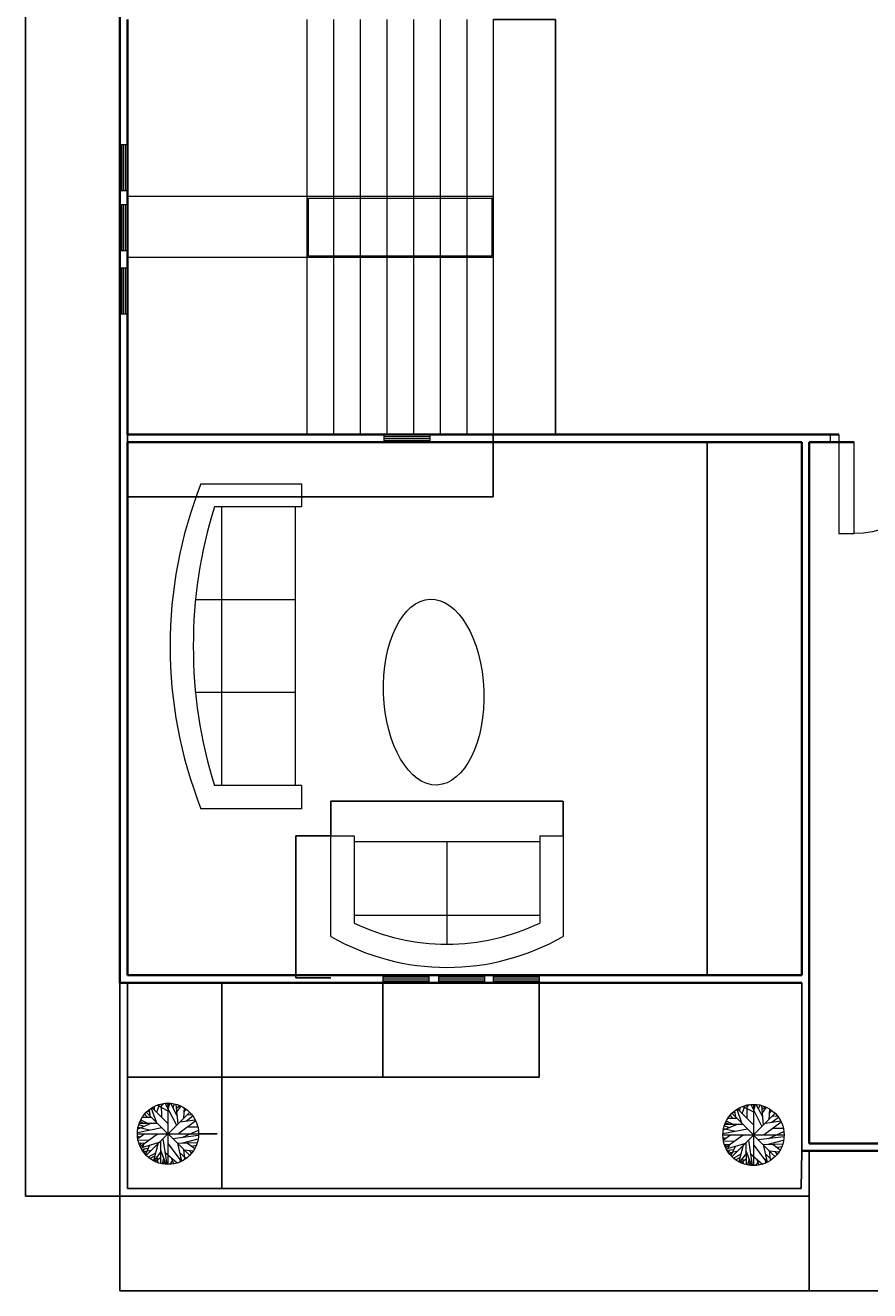
# Model space of a CAD drawing. Units: millimetres. Extents: x 1194 to 22780, y 83 to 13378.
# Tile 4 of 6: x 12489 to 18030, y 136 to 8443. Entities that reach past the tile are written whole.
import ezdxf

# ---------------------------------------------------------------- set-up
doc = ezdxf.new("R2010")
doc.units = ezdxf.units.MM
for name, color, linetype, lineweight in [('A-ANNO-DIMS', 2, 'Continuous', 18), ('A-DOOR', 3, 'Continuous', 18), ('A-FLOR-STRS', 7, 'Continuous', 18), ('A-FURN', 8, 'Continuous', 18), ('A-GLAZ', 4, 'Continuous', 18), ('A-WALL', 7, 'Continuous', 35), ('A-WALL-PRPT', 7, 'Continuous', 25), ('L-PLNT', 3, 'Continuous', 13)]:
    doc.layers.add(name, color=color, linetype=linetype, lineweight=lineweight)
doc.styles.get("Standard").update_dxf_attribs({"font": 'arial.ttf'})
doc.dimstyles.get("Standard").update_dxf_attribs({"dimtxt": 0.18, "dimasz": 0.18, "dimexe": 0.18, "dimexo": 0.0625, "dimgap": 0.09, "dimtad": 0, "dimtih": 1, "dimtoh": 1, "dimdec": 4, "dimzin": 0, "dimdsep": 46, "dimtxsty": 'Standard', "dimcen": 0.09, "dimadec": 0, "dimazin": 0, "dimtfac": 1, "dimtdec": 4, "dimtofl": 0, "dimtmove": 0, "dimatfit": 3, "dimfxl": 1, "dimtolj": 1, "dimtzin": 0, "dimarcsym": 0})

# ---------------------------------------------------------------- blocks, each defined once
blk = doc.blocks.new('Window - Wood Frame 36 in. Wide plan')
for p, q in [((0, 6), (0, 0)), ((0, 4.5), (36, 4.5)), ((0, 3), (36, 3)), ((0, 1.5), (36, 1.5)), ((36, 6), (36, 0))]:
    blk.add_line(p, q)
blk = doc.blocks.new('Sofa - Roundback 7 ft.')
for p, q in [((-12.00002, -32.4421), (-12.00003, -6.5971)), ((11.99997, -32.4421), (11.99998, -6.5971)), ((-36.000027, -34), (-36.000027, -11.4696)), ((35.99998, -34), (35.99998, -11.4696)), ((-35.999844, -13.3819), (35.9998, -13.3819)), ((-36.000027, -32.4421), (35.99998, -32.4421))]:
    blk.add_line(p, q)
for points in [[(-36.000027, -34), (-42.000027, -34), (-42.000027, -8)], [(41.99998, -8), (41.99998, -34), (35.99998, -34)]]:
    blk.add_lwpolyline(points)
for centre, radius, start, end in [((0, -114.25), 114.25, 68.43141, 111.5686), ((-0.00001, -127.1968), 121.1968, 72.72033, 107.2797)]:
    blk.add_arc(centre, radius, start, end)
blk = doc.blocks.new('Sofa - Roundback Loveseat 5 ft.')
for p, q in [((0, -32.44198), (0, -5.99998)), ((-24, -33.99998), (-24, -11.46958)), ((24.00004, -33.99998), (24.00004, -11.46958)), ((-23.9998, -13.38178), (23.99986, -13.38178)), ((-24, -32.44198), (24.00004, -32.44198))]:
    blk.add_line(p, q)
for points in [[(-24, -33.99998), (-30, -33.99998), (-30, -7.99998)], [(30.00004, -7.99998), (30.00004, -33.99998), (24.00004, -33.99998)]]:
    blk.add_lwpolyline(points)
for centre, radius, start, end in [((0, -60.24998), 60.24998, 60.13715, 119.8628), ((0, -61.38438), 55.38444, 64.32083, 115.6792)]:
    blk.add_arc(centre, radius, start, end)
blk = doc.blocks.new('Tree - deciduous plan')
for p, q in [((-32.6092, 50.4264), (-23.2782, 23.5674)), ((-31.2008, 51.1035), (-0.2149, 20.1818)), ((-26.4472, 46.5894), (-26.2712, 53.8116)), ((-22.0458, 42.0753), (-16.5881, 57.6486)), ((-21.1656, 55.8436), (-0.0388, 45.0094)), ((-12.5388, 54.9406), (-7.9613, 59.4546)), ((-12.3627, 32.1443), (-12.5388, 58.7776)), ((-5.3205, 59.6806), (16.5105, 16.7963)), ((2.426, 54.9406), (-1.4472, 59.9056)), ((0, 59.9996), (0, -60)), ((0.4894, 48.6208), (3.6584, 59.6806)), ((18.2711, 35.5298), (5.419, 59.6806)), ((9.8203, 51.5549), (12.8133, 58.5516)), ((19.6795, 19.5047), (16.3344, 57.6486)), ((17.0387, 51.1035), (23.2006, 55.1666)), ((17.7429, 43.6552), (25.4894, 54.2636)), ((31.6513, 50.8778), (30.2429, 30.5643)), ((-53.2078, 27.4044), (-40.1797, 20.859)), ((-49.8627, 32.8214), (-32.7853, 32.8214)), ((-45.8134, 38.2383), (-40.5318, 33.0471)), ((-43.8768, 36.4326), (-44.405, 40.2696)), ((42, 42), (-42, -42)), ((42, -42), (-42, 42)), ((-40.1797, 44.558), (-36.4825, 43.2038)), ((-37.0107, 47.0408), (-35.25, 35.5298)), ((54.3626, 25.3731), (20.9119, 0.3198)), ((23.3767, 23.3417), (53.3063, 27.4044)), ((31.1232, 42.5267), (35.8767, 48.1693)), ((36.2288, 25.1474), (48.9049, 35.0784)), ((37.1091, 37.1098), (46.6161, 37.5612)), ((-59.7219, 2.8025), (-12.0106, 12.0565)), ((-32.2571, 20.6333), (-59.1937, 9.348)), ((-58.6656, 12.7336), (-35.9543, 7.5424)), ((-57.081, 17.9248), (-47.0458, 14.7649)), ((-56.0247, 20.859), (-20.8134, 20.859)), ((-54.7923, 24.4702), (-47.75, 21.0847)), ((-54.6162, -24.7335), (-20.2853, 0.0941)), ((29.3626, -6.6771), (59.4682, 7.091)), ((38.5175, 13.4107), (58.2359, 13.6364)), ((-60, 0), (60, 0)), ((-59.7219, -4.8714), (-54.2641, -6.6771)), ((-45.2853, -0.1316), (-59.0177, -10.0627)), ((-58.4895, -12.3197), (-36.4825, -11.6426)), ((-57.081, -18.4138), (-45.2853, -17.9624)), ((-52.6797, -18.188), (-55.4966, -22.0251)), ((-53.2078, -27.442), (-16.7641, -16.6081)), ((-47.2219, -19.3166), (-50.2148, -26.3135)), ((-35.9543, -22.4765), (-44.0529, -40.5329)), ((-19.9331, -20.2194), (-28.5599, -52.721)), ((-14.8275, -15.0282), (-14.6515, -57.6865)), ((-10.074, -10.0627), (-2.5036, -59.7178)), ((-0.0388, -19.0909), (25.8415, -53.8495)), ((9.2922, -9.1598), (59.6443, -2.8401)), ((18.6232, -18.6394), (26.7218, -53.3981)), ((18.7992, -18.6394), (57.3556, -17.2853)), ((26.3697, -18.4138), (58.9401, -9.8369)), ((38.1654, -18.188), (52.426, -29.0219)), ((45.9119, -24.0564), (55.595, -22.2508)), ((-38.9472, -29.0219), (-51.4472, -30.6018)), ((-46.5177, -30.1504), (-49.5106, -33.536)), ((-32.4331, -32.4075), (-48.1021, -35.5674)), ((-43.7008, -34.6645), (-46.6937, -37.373)), ((-24.6867, -37.8244), (-38.7712, -45.7241)), ((-26.2712, -43.9185), (-34.7219, -48.6583)), ((-14.6515, -36.2445), (-27.6797, -52.9467)), ((-14.6515, -47.3041), (-25.0388, -54.3009)), ((-21.5177, -45.4984), (-19.9331, -56.1065)), ((-14.6515, -32.1818), (-3.912, -59.4922)), ((-8.4895, -47.5298), (-11.4825, -58.5893)), ((-6.2008, -36.2445), (17.919, -57.0094)), ((5.9471, -46.6269), (10.5246, -58.5893)), ((22.8485, -36.4702), (35.3485, -48.4326)), ((24.7852, -44.8213), (23.0246, -54.978)), ((30.419, -30.1504), (32.3556, -50.0125)), ((31.4753, -31.279), (49.6091, -33.3103)), ((41.5105, -32.6332), (46.088, -38.0501)), ((-6.3768, -52.721), (-9.3698, -58.815)), ((8.4119, -53.1724), (3.8344, -59.4922))]:
    blk.add_line(p, q)
blk.add_circle((0, 0), 60)
blk = doc.blocks.new('DOOR-SWING-600')
for p, q in [((0, 0), (0, 600)), ((0, 600), (100, 600)), ((100, 600), (100, 0))]:
    blk.add_line(p, q)
blk.add_arc((100, 0), 600, 0, 90)
blk = doc.blocks.new('STAIR-DUPLEX-FLIGHT')
for p, q in [((1177, 2725.9), (1177, 0)), ((1351.8, 2725.9), (1351.8, 0)), ((1526.7, 2725.9), (1526.7, 0)), ((1701.5, 2725.9), (1701.5, 0)), ((1876.4, 2725.9), (1876.4, 0)), ((2051.2, 2725.9), (2051.2, 0)), ((2226.1, 2725.9), (2226.1, 0)), ((2400.9, 2725.9), (2400.9, 0)), ((1177, 1562.9), (0, 1562.9)), ((2400.9, 1562.9), (1177, 1562.9)), ((1187, 1552.9), (2390.9, 1552.9)), ((1187, 1172.9), (1187, 1552.9)), ((2390.9, 1552.9), (2390.9, 1172.9)), ((2400.9, 1362.9), (2400.9, 1562.9)), ((2390.9, 1172.9), (1187, 1172.9)), ((2400.9, 1162.9), (0, 1162.9))]:
    blk.add_line(p, q)
blk = doc.blocks.new('*D33')
at = {"layer": 'A-ANNO-DIMS', "color": 0, "lineweight": -2, "transparency": 16777216}
for p, q in [((14493.6, 3121.8), (14493.6, 3350.5)), ((14493.8, 3350.4), (15254.3, 3350.4)), ((16017.4, 3350.4), (15257, 3350.4)), ((16017.6, 3121.8), (16017.6, 3350.5))]:
    blk.add_line(p, q, dxfattribs=at)
at = {"layer": 'A-ANNO-DIMS', "color": 0, "transparency": 16777216}
for points in [[(14493.8, 3350.4), (14493.8, 3350.3), (14493.6, 3350.4)], [(16017.4, 3350.4), (16017.4, 3350.3), (16017.6, 3350.4)]]:
    blk.add_solid(points, dxfattribs=at)
at = {"layer": 'Defpoints', "color": 0, "transparency": 16777216}
for p in [(14493.6, 3350.4), (14493.6, 3121.8), (16017.6, 3121.8)]:
    blk.add_point(p, dxfattribs=at)
at = {"layer": 'A-ANNO-DIMS', "color": 0, "transparency": 16777216, "insert": (15255.6, 3350.4), "char_height": 0.18, "attachment_point": 5}
blk.add_mtext('\\A1;LOVESEAT 1524 TYP.', dxfattribs=at)
blk = doc.blocks.new('*D34')
at = {"layer": 'A-ANNO-DIMS', "color": 0, "lineweight": -2, "transparency": 16777216}
for p, q in [((14493.6, 3121.8), (14264.8, 3121.8)), ((14265, 3121.6), (14265, 2656.3)), ((14265, 2190.6), (14265, 2655.9)), ((14493.6, 2190.4), (14264.8, 2190.4))]:
    blk.add_line(p, q, dxfattribs=at)
at = {"layer": 'A-ANNO-DIMS', "color": 0, "transparency": 16777216}
for points in [[(14265, 3121.6), (14265, 3121.6), (14265, 3121.8)], [(14265, 2190.6), (14265, 2190.6), (14265, 2190.4)]]:
    blk.add_solid(points, dxfattribs=at)
at = {"layer": 'Defpoints', "color": 0, "transparency": 16777216}
for p in [(14493.6, 3121.8), (14265, 2190.4), (14493.6, 2190.4)]:
    blk.add_point(p, dxfattribs=at)
at = {"layer": 'A-ANNO-DIMS', "color": 0, "transparency": 16777216, "insert": (14265, 2656.1), "char_height": 0.18, "attachment_point": 5}
blk.add_mtext('\\A1;931 TYP.', dxfattribs=at)
blk = doc.blocks.new('*D39')
at = {"layer": 'A-ANNO-DIMS', "color": 0, "lineweight": -2, "transparency": 16777216}
for p, q in [((15560.2, 8481.6), (15969.2, 8481.6)), ((15969, 8481.5), (15969, 7118.9)), ((15969, 5756), (15969, 7118.5)), ((15560.2, 5755.8), (15969.2, 5755.8))]:
    blk.add_line(p, q, dxfattribs=at)
at = {"layer": 'A-ANNO-DIMS', "color": 0, "transparency": 16777216}
for points in [[(15969, 8481.5), (15969, 8481.5), (15969, 8481.6)], [(15969, 5756), (15969, 5756), (15969, 5755.8)]]:
    blk.add_solid(points, dxfattribs=at)
at = {"layer": 'Defpoints', "color": 0, "transparency": 16777216}
for p in [(15560.1, 8481.6), (15969, 8481.6), (15560.1, 5755.8)]:
    blk.add_point(p, dxfattribs=at)
at = {"layer": 'A-ANNO-DIMS', "color": 0, "transparency": 16777216, "insert": (15969, 7118.7), "char_height": 0.18, "attachment_point": 5}
blk.add_mtext('\\A1;STAIR 2726 TYP.', dxfattribs=at)
blk = doc.blocks.new('*D40')
at = {"layer": 'A-ANNO-DIMS', "color": 0, "lineweight": -2, "transparency": 16777216}
for p, q in [((13159.2, 5755.7), (13159.2, 5346.7)), ((15560.1, 5755.7), (15560.1, 5346.7)), ((13159.4, 5346.9), (14359, 5346.9)), ((15559.9, 5346.9), (14360.3, 5346.9))]:
    blk.add_line(p, q, dxfattribs=at)
at = {"layer": 'A-ANNO-DIMS', "color": 0, "transparency": 16777216}
for points in [[(13159.4, 5346.9), (13159.4, 5346.9), (13159.2, 5346.9)], [(15559.9, 5346.9), (15559.9, 5346.9), (15560.1, 5346.9)]]:
    blk.add_solid(points, dxfattribs=at)
at = {"layer": 'Defpoints', "color": 0, "transparency": 16777216}
for p in [(13159.2, 5755.8), (15560.1, 5755.8), (15560.1, 5346.9)]:
    blk.add_point(p, dxfattribs=at)
at = {"layer": 'A-ANNO-DIMS', "color": 0, "transparency": 16777216, "insert": (14359.7, 5346.9), "char_height": 0.18, "attachment_point": 5}
blk.add_mtext('\\A1;2401 TYP.', dxfattribs=at)
blk = doc.blocks.new('*D73')
at = {"layer": 'A-ANNO-DIMS', "color": 0, "lineweight": -2, "transparency": 16777216}
for p, q in [((13109.1, 12755.8), (12488.7, 12755.8)), ((12488.9, 12755.6), (12488.9, 6756)), ((12488.9, 756), (12488.9, 6755.6)), ((13109.1, 755.8), (12488.7, 755.8))]:
    blk.add_line(p, q, dxfattribs=at)
at = {"layer": 'A-ANNO-DIMS', "color": 0, "transparency": 16777216}
for points in [[(12488.8, 12755.6), (12488.9, 12755.6), (12488.9, 12755.8)], [(12488.8, 756), (12488.9, 756), (12488.9, 755.8)]]:
    blk.add_solid(points, dxfattribs=at)
at = {"layer": 'Defpoints', "color": 0, "transparency": 16777216}
for p in [(12488.9, 12755.8), (13109.2, 12755.8), (13109.2, 755.8)]:
    blk.add_point(p, dxfattribs=at)
at = {"layer": 'A-ANNO-DIMS', "color": 0, "transparency": 16777216, "insert": (12488.9, 6755.8), "char_height": 0.18, "attachment_point": 5}
blk.add_mtext('\\A1;12000', dxfattribs=at)
blk = doc.blocks.new('*D74')
at = {"layer": 'A-ANNO-DIMS', "color": 0, "lineweight": -2, "transparency": 16777216}
for p, q in [((13109.2, 755.8), (13109.2, 135.6)), ((17634.2, 755.8), (17634.2, 135.6)), ((13109.4, 135.8), (15371.3, 135.8)), ((17634, 135.8), (15372.1, 135.8))]:
    blk.add_line(p, q, dxfattribs=at)
at = {"layer": 'A-ANNO-DIMS', "color": 0, "transparency": 16777216}
for points in [[(13109.4, 135.8), (13109.4, 135.8), (13109.2, 135.8)], [(17634, 135.8), (17634, 135.8), (17634.2, 135.8)]]:
    blk.add_solid(points, dxfattribs=at)
at = {"layer": 'Defpoints', "color": 0, "transparency": 16777216}
for p in [(13109.2, 755.8), (17634.2, 755.8), (17634.2, 135.8)]:
    blk.add_point(p, dxfattribs=at)
at = {"layer": 'A-ANNO-DIMS', "color": 0, "transparency": 16777216, "insert": (15371.7, 135.8), "char_height": 0.18, "attachment_point": 5}
blk.add_mtext('\\A1;4525', dxfattribs=at)
blk = doc.blocks.new('*D75')
at = {"layer": 'A-ANNO-DIMS', "color": 0, "lineweight": -2, "transparency": 16777216}
for p, q in [((22159.2, 1052.8), (22159.2, 135.6)), ((17634.2, 755.8), (17634.2, 135.6)), ((17634.4, 135.8), (19896.3, 135.8)), ((22159, 135.8), (19897.1, 135.8))]:
    blk.add_line(p, q, dxfattribs=at)
at = {"layer": 'A-ANNO-DIMS', "color": 0, "transparency": 16777216}
for points in [[(17634.4, 135.8), (17634.4, 135.8), (17634.2, 135.8)], [(22159, 135.8), (22159, 135.8), (22159.2, 135.8)]]:
    blk.add_solid(points, dxfattribs=at)
at = {"layer": 'Defpoints', "color": 0, "transparency": 16777216}
for p in [(22159.2, 1052.8), (17634.2, 755.8), (22159.2, 135.8)]:
    blk.add_point(p, dxfattribs=at)
at = {"layer": 'A-ANNO-DIMS', "color": 0, "transparency": 16777216, "insert": (19896.7, 135.8), "char_height": 0.18, "attachment_point": 5}
blk.add_mtext('\\A1;4525', dxfattribs=at)
blk = doc.blocks.new('*D84')
at = {"layer": 'A-ANNO-DIMS', "color": 0, "lineweight": -2, "transparency": 16777216}
for p, q in [((17584.1, 5705.8), (16964, 5705.8)), ((16964.2, 5705.6), (16964.2, 3957)), ((16964.2, 2207.9), (16964.2, 3956.6)), ((17584.1, 2207.8), (16964, 2207.8))]:
    blk.add_line(p, q, dxfattribs=at)
at = {"layer": 'A-ANNO-DIMS', "color": 0, "transparency": 16777216}
for points in [[(16964.2, 5705.6), (16964.2, 5705.6), (16964.2, 5705.8)], [(16964.2, 2207.9), (16964.2, 2207.9), (16964.2, 2207.8)]]:
    blk.add_solid(points, dxfattribs=at)
at = {"layer": 'Defpoints', "color": 0, "transparency": 16777216}
for p in [(16964.2, 5705.8), (17584.2, 5705.8), (17584.2, 2207.8)]:
    blk.add_point(p, dxfattribs=at)
at = {"layer": 'A-ANNO-DIMS', "color": 0, "transparency": 16777216, "insert": (16964.2, 3956.8), "char_height": 0.18, "attachment_point": 5}
blk.add_mtext('\\A1;3498', dxfattribs=at)
blk = doc.blocks.new('*D86')
at = {"layer": 'A-ANNO-DIMS', "color": 0, "lineweight": -2, "transparency": 16777216}
for p, q in [((13159.3, 2157.8), (13779.4, 2157.8)), ((13779.2, 2157.6), (13779.2, 1482)), ((13779.2, 806), (13779.2, 1481.6)), ((13159.3, 805.8), (13779.4, 805.8))]:
    blk.add_line(p, q, dxfattribs=at)
at = {"layer": 'A-ANNO-DIMS', "color": 0, "transparency": 16777216}
for points in [[(13779.2, 2157.6), (13779.2, 2157.6), (13779.2, 2157.8)], [(13779.2, 806), (13779.2, 806), (13779.2, 805.8)]]:
    blk.add_solid(points, dxfattribs=at)
at = {"layer": 'Defpoints', "color": 0, "transparency": 16777216}
for p in [(13159.2, 2157.8), (13159.2, 805.8), (13779.2, 805.8)]:
    blk.add_point(p, dxfattribs=at)
at = {"layer": 'A-ANNO-DIMS', "color": 0, "transparency": 16777216, "insert": (13779.2, 1481.8), "char_height": 0.18, "attachment_point": 5}
blk.add_mtext('\\A1;1352', dxfattribs=at)
blk = doc.blocks.new('*D87')
at = {"layer": 'A-ANNO-DIMS', "color": 0, "lineweight": -2, "transparency": 16777216}
for p, q in [((13159.2, 2157.7), (13159.1, 1537.6)), ((14835.9, 2157.4), (14835.8, 1537.3)), ((13159.3, 1537.8), (13997, 1537.6)), ((14835.6, 1537.4), (13997.9, 1537.6))]:
    blk.add_line(p, q, dxfattribs=at)
at = {"layer": 'A-ANNO-DIMS', "color": 0, "transparency": 16777216}
for points in [[(13159.3, 1537.8), (13159.3, 1537.7), (13159.1, 1537.8)], [(14835.6, 1537.5), (14835.6, 1537.4), (14835.8, 1537.4)]]:
    blk.add_solid(points, dxfattribs=at)
at = {"layer": 'Defpoints', "color": 0, "transparency": 16777216}
for p in [(13159.2, 2157.8), (14835.9, 2157.4), (13159.1, 1537.8)]:
    blk.add_point(p, dxfattribs=at)
at = {"layer": 'A-ANNO-DIMS', "color": 0, "transparency": 16777216, "insert": (13997.5, 1537.6), "char_height": 0.18, "attachment_point": 5}
blk.add_mtext('\\A1;1676.7', dxfattribs=at)
blk = doc.blocks.new('*D88')
at = {"layer": 'A-ANNO-DIMS', "color": 0, "lineweight": -2, "transparency": 16777216}
for p, q in [((14835.9, 2157.4), (14835.9, 1537.3)), ((15861.4, 2157.4), (15861.4, 1537.3)), ((14836.1, 1537.4), (15348.2, 1537.4)), ((15861.2, 1537.4), (15349.1, 1537.4))]:
    blk.add_line(p, q, dxfattribs=at)
at = {"layer": 'A-ANNO-DIMS', "color": 0, "transparency": 16777216}
for points in [[(14836.1, 1537.5), (14836.1, 1537.4), (14835.9, 1537.4)], [(15861.2, 1537.5), (15861.2, 1537.4), (15861.4, 1537.4)]]:
    blk.add_solid(points, dxfattribs=at)
at = {"layer": 'Defpoints', "color": 0, "transparency": 16777216}
for p in [(14835.9, 2157.4), (15861.4, 2157.4), (14835.9, 1537.4)]:
    blk.add_point(p, dxfattribs=at)
at = {"layer": 'A-ANNO-DIMS', "color": 0, "transparency": 16777216, "insert": (15348.7, 1537.4), "char_height": 0.18, "attachment_point": 5}
blk.add_mtext('\\A1;1025.5', dxfattribs=at)
blk = doc.blocks.new('*D99')
at = {"layer": 'A-ANNO-DIMS', "color": 0, "lineweight": -2, "transparency": 16777216}
for p, q in [((13424.9, 1165.5), (13424.9, 1165.7)), ((13424.9, 1165.6), (13425, 1165.6)), ((13746.8, 1165.6), (13626.3, 1165.6))]:
    blk.add_line(p, q, dxfattribs=at)
at = {"layer": 'A-ANNO-DIMS', "color": 0, "transparency": 16777216}
blk.add_solid([(13626.3, 1165.6), (13626.3, 1165.6), (13626.1, 1165.6)], dxfattribs=at)
at = {"layer": 'Defpoints', "color": 0, "transparency": 16777216}
for p in [(13223.8, 1165.6), (13626.1, 1165.6)]:
    blk.add_point(p, dxfattribs=at)
at = {"layer": 'A-ANNO-DIMS', "color": 0, "transparency": 16777216, "insert": (13747.5, 1165.6), "char_height": 0.18, "attachment_point": 5}
blk.add_mtext('\\A1;2X ∅402.3', dxfattribs=at)

msp = doc.modelspace()

# ---------------------------------------------------------------- linework, layer by layer
at = {"layer": 'A-DOOR'}
for p, q in [((17773.789, 5705.774), (17773.789, 5755.774)), ((17773.789, 5705.774), (17773.789, 5755.774)), ((17773.789, 5755.774), (17827.474, 5755.774)), ((17827.474, 5755.774), (17827.474, 5705.774)), ((17773.789, 5705.774), (17927.474, 5705.774))]:
    msp.add_line(p, q, dxfattribs=at)
at = {"layer": 'A-FURN'}
msp.add_ellipse((15168.291, 4065.558), major_axis=(-22.607, 609.897), ratio=0.53984917, dxfattribs=at)
at = {"layer": 'A-WALL'}
for p, q in [((13109.207, 12730.774), (13109.207, 2157.764)), ((13159.207, 8481.636), (13159.207, 5755.774)), ((16134.207, 5755.774), (13159.207, 5755.774)), ((16134.207, 5755.774), (16609.207, 5755.774)), ((16609.207, 5755.774), (16659.207, 5755.774)), ((16659.207, 5755.774), (17827.474, 5755.774)), ((13159.207, 5705.774), (13159.207, 2207.764)), ((16134.207, 5705.774), (13159.207, 5705.774)), ((16134.207, 5705.774), (16609.207, 5705.774)), ((16609.207, 5705.774), (17584.207, 5705.774)), ((17584.207, 5655.774), (17584.207, 5705.774)), ((17584.207, 5655.774), (17584.207, 2207.764)), ((17634.207, 5705.774), (17634.207, 3305.774)), ((17634.207, 1102.813), (17634.207, 5705.774)), ((17634.207, 5705.774), (17927.474, 5705.774)), ((13159.207, 2207.764), (17584.207, 2207.764)), ((17584.207, 2157.764), (13109.207, 2157.764)), ((17634.207, 1102.813), (22109.207, 1102.813)), ((17584.207, 1052.813), (22159.207, 1052.813))]:
    msp.add_line(p, q, dxfattribs=at)
at = {"layer": 'A-WALL-PRPT'}
for p, q in [((13109.207, 2157.764), (13109.207, 755.817)), ((13159.207, 2157.764), (13159.207, 805.817)), ((17584.207, 2157.764), (17584.207, 1860.725)), ((17584.207, 1860.725), (17584.207, 1810.725)), ((17584.207, 1810.725), (17584.207, 1052.813)), ((17580.802, 805.817), (17584.207, 1052.813)), ((17584.207, 1052.813), (17634.207, 1052.813)), ((17634.207, 1052.813), (17634.207, 755.817)), ((13141.49, 755.817), (13109.207, 755.817)), ((13109.207, 755.817), (17580.112, 755.817)), ((17584.207, 755.817), (13109.207, 755.817)), ((13159.207, 805.817), (17580.802, 805.817)), ((17634.207, 755.817), (17580.112, 755.817))]:
    msp.add_line(p, q, dxfattribs=at)

# ---------------------------------------------------------------- block references
at = {"layer": 'A-DOOR', "extrusion": (0, 0, -1), "zscale": -1, "rotation": 180}
msp.add_blockref('DOOR-SWING-600', (-17827.475, 5705.774), dxfattribs=at)
at = {"layer": 'A-FLOR-STRS'}
msp.add_blockref('STAIR-DUPLEX-FLIGHT', (13159.207, 5755.774), dxfattribs=at)
at = {"layer": 'A-FURN'}
for name, p, xscale, yscale, zscale, rotation in [('Sofa - Roundback 7 ft.', (13438.36, 4366.975), 25.40000000000003, 25.40000000000003, 25.40000000000003, 90.00000812057576), ('Sofa - Roundback Loveseat 5 ft.', (15255.618, 2258.158), 25.4, 25.4, 25.4, 180)]:
    msp.add_blockref(name, p, dxfattribs=dict(at, xscale=xscale, yscale=yscale, zscale=zscale, rotation=rotation))
at = {"layer": 'A-GLAZ', "xscale": 8.388003104210137, "yscale": 8.388003104210137, "zscale": 8.388003104210137, "rotation": 90}
for p in [(13159.207, 7358.738), (13159.207, 6964.303), (13159.207, 6549.98)]:
    msp.add_blockref('Window - Wood Frame 36 in. Wide plan', p, dxfattribs=at)
at = {"layer": 'A-GLAZ', "xscale": 8.388003104210137, "yscale": 8.388003104210137, "zscale": 8.388003104210137}
for p in [(14842.354, 5705.446), (14835.945, 2157.436), (15200.577, 2157.436), (15559.446, 2157.436)]:
    msp.add_blockref('Window - Wood Frame 36 in. Wide plan', p, dxfattribs=at)
at = {"layer": 'L-PLNT', "xscale": 3.352694576473469, "yscale": 3.352694576473469, "zscale": 3.352694576473469}
for p in [(13424.948, 1165.591), (17267.777, 1157.931)]:
    msp.add_blockref('Tree - deciduous plan', p, dxfattribs=at)

# ---------------------------------------------------------------- dimensions: what is measured, and where the dimension line sits
at = {"layer": 'A-ANNO-DIMS'}
for base, p1, p2, angle, override, picture, middle in [((12488.879, 12755.774), (13109.207, 755.817), (13109.207, 12755.774), 90, {"dimdec": 0, "dimlfac": 1, "dimrnd": 0, "dimzin": 0, "dimdsep": 46, "dimlunit": 2}, '*D73', (12488.879, 6755.796)), ((16964.207, 5705.774), (17584.207, 2207.764), (17584.207, 5705.774), 90, {"dimdec": 0, "dimlfac": 1, "dimrnd": 0, "dimzin": 0, "dimdsep": 46, "dimlunit": 2}, '*D84', (16964.207, 3956.769)), ((13159.085, 1537.764), (14835.945, 2157.436), (13159.207, 2157.764), 179.9887913, {"dimdec": 1, "dimlfac": 1, "dimrnd": 0, "dimzin": 0, "dimdsep": 46, "dimlunit": 2}, '*D87', (13997.455, 1537.6)), ((13779.207, 805.817), (13159.207, 2157.764), (13159.207, 805.817), 270, {"dimdec": 0, "dimlfac": 1, "dimrnd": 0, "dimzin": 0, "dimdsep": 46, "dimlunit": 2}, '*D86', (13779.207, 1481.791)), ((14835.945, 1537.436), (15861.414, 2157.436), (14835.945, 2157.436), 180, {"dimdec": 1, "dimlfac": 1, "dimrnd": 0, "dimzin": 0, "dimdsep": 46, "dimlunit": 2}, '*D88', (15348.679, 1537.436))]:
    dim = msp.add_linear_dim(base=base, p1=p1, p2=p2, angle=angle, dimstyle='Standard', override=override, dxfattribs=at)
    dim.commit()
    dim.dimension.update_dxf_attribs({"geometry": picture, "text_midpoint": middle})
for base, p1, p2, angle, text, picture, middle in [((15968.995, 8481.636), (15560.115, 5755.774), (15560.115, 8481.636), 90, 'STAIR <> TYP.', '*D39', (15968.995, 7118.705)), ((14493.617, 3350.357), (16017.618, 3121.757), (14493.617, 3121.757), 180, 'LOVESEAT <> TYP.', '*D33', (15255.617, 3350.357)), ((14265.017, 2190.424), (14493.617, 3121.757), (14493.617, 2190.424), 270, '<> TYP.', '*D34', (14265.017, 2656.091))]:
    dim = msp.add_linear_dim(base=base, p1=p1, p2=p2, angle=angle, text=text, dimstyle='Standard', override={"dimdec": 0, "dimlfac": 1, "dimrnd": 0, "dimzin": 0, "dimdsep": 46, "dimlunit": 2}, dxfattribs=at)
    dim.commit()
    dim.dimension.update_dxf_attribs({"geometry": picture, "text_midpoint": middle})
dim = msp.add_linear_dim(base=(15560.115, 5346.894), p1=(13159.207, 5755.774), p2=(15560.115, 5755.774), text='<> TYP.', dimstyle='Standard', override={"dimdec": 0, "dimlfac": 1, "dimrnd": 0, "dimzin": 0, "dimdsep": 46, "dimlunit": 2}, dxfattribs=at)
dim.commit()
dim.dimension.update_dxf_attribs({"geometry": '*D40', "text_midpoint": (14359.661, 5346.894)})
dim = msp.add_diameter_dim_2p(p1=(13223.786, 1165.591), p2=(13626.11, 1165.591), text='2X <>', dimstyle='Standard', override={"dimdec": 1, "dimlfac": 1, "dimrnd": 0, "dimzin": 0, "dimdsep": 46, "dimlunit": 2}, dxfattribs=at)
dim.commit()
dim.dimension.update_dxf_attribs({"geometry": '*D99', "text_midpoint": (13746.807, 1165.591), "dimtype": 163})
for base, p1, p2, picture, middle in [((22159.207, 135.817), (17634.207, 755.817), (22159.207, 1052.813), '*D75', (19896.707, 135.817)), ((17634.207, 135.817), (13109.207, 755.817), (17634.207, 755.817), '*D74', (15371.707, 135.817))]:
    dim = msp.add_linear_dim(base=base, p1=p1, p2=p2, dimstyle='Standard', override={"dimdec": 0, "dimlfac": 1, "dimrnd": 0, "dimzin": 0, "dimdsep": 46, "dimlunit": 2}, dxfattribs=at)
    dim.commit()
    dim.dimension.update_dxf_attribs({"geometry": picture, "text_midpoint": middle})

doc.saveas('drawing.dxf')
